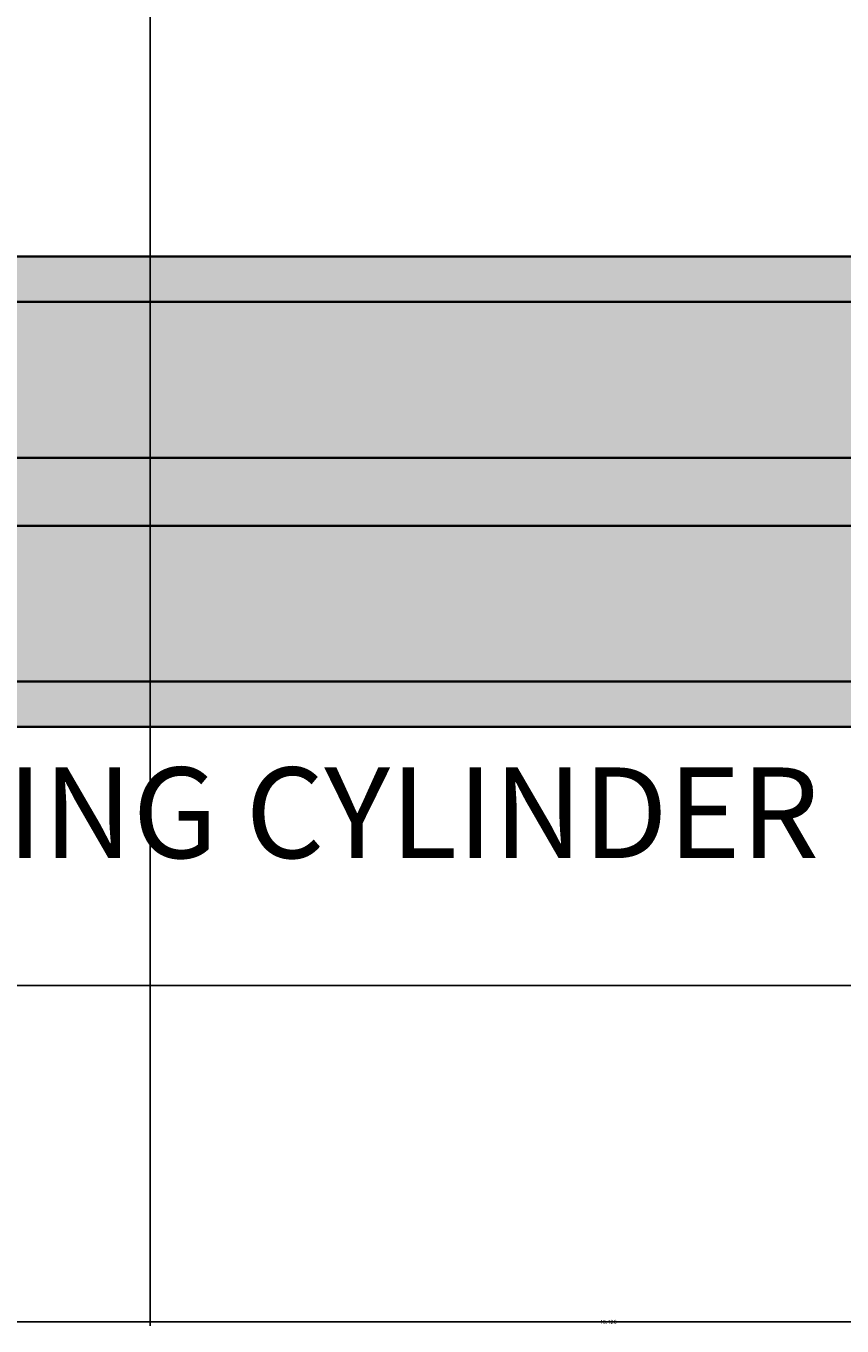
# Model space of a CAD drawing. Units: millimetres. Extents: x -11 to 280, y -4 to 208.
# Tile 28 of 55: x 186 to 222, y -4 to 54. Entities that reach past the tile are written whole.
import ezdxf

# ---------------------------------------------------------------- set-up
doc = ezdxf.new("R2010")
doc.units = ezdxf.units.MM
for name, color, linetype, lineweight in [('M-ANNO-TEXT', 7, 'Continuous', 18), ('M-DIMS', 2, 'Continuous', 18), ('M-HYDR-CYL', 7, 'Continuous', 35), ('M-HYDR-CYL-PATT', 252, 'Continuous', 13)]:
    doc.layers.add(name, color=color, linetype=linetype, lineweight=lineweight)
doc.styles.get("Standard").update_dxf_attribs({"font": 'arial.ttf'})
doc.dimstyles.get("Standard").update_dxf_attribs({"dimtxt": 0.18, "dimasz": 0.18, "dimexe": 0.18, "dimexo": 0.0625, "dimgap": 0.09, "dimtad": 0, "dimtih": 1, "dimtoh": 1, "dimdec": 4, "dimzin": 0, "dimdsep": 46, "dimtxsty": 'Standard', "dimcen": 0.09, "dimadec": 0, "dimazin": 0, "dimtfac": 1, "dimtdec": 4, "dimtofl": 0, "dimtmove": 0, "dimatfit": 3, "dimfxl": 1, "dimtolj": 1, "dimtzin": 0, "dimarcsym": 0})

# ---------------------------------------------------------------- blocks, each defined once
blk = doc.blocks.new('*D4')
at = {"layer": 'Defpoints', "color": 0, "transparency": 16777216}
for p in [(4.763, 84.426), (266.035, 51.733), (266.035, -3.415)]:
    blk.add_point(p, dxfattribs=at)
at = {"layer": 'M-DIMS', "color": 0, "lineweight": -2, "transparency": 16777216}
for p, q in [((4.763, 84.364), (4.763, -3.595)), ((266.035, 51.67), (266.035, -3.595)), ((4.943, -3.415), (134.934, -3.415)), ((265.855, -3.415), (135.864, -3.415))]:
    blk.add_line(p, q, dxfattribs=at)
at = {"layer": 'M-DIMS', "color": 0, "transparency": 16777216}
for points in [[(4.943, -3.385), (4.943, -3.445), (4.763, -3.415)], [(265.855, -3.385), (265.855, -3.445), (266.035, -3.415)]]:
    blk.add_solid(points, dxfattribs=at)
at = {"layer": 'M-DIMS', "color": 0, "transparency": 16777216, "insert": (135.399, -3.415), "char_height": 0.18, "attachment_point": 5}
blk.add_mtext('\\A1;261.27', dxfattribs=at)
blk = doc.blocks.new('*D5')
at = {"layer": 'Defpoints', "color": 0, "transparency": 16777216}
for p in [(24.759, 192.645), (-10.087, 11.435), (261.686, 11.435)]:
    blk.add_point(p, dxfattribs=at)
at = {"layer": 'M-DIMS', "color": 0, "lineweight": -2, "transparency": 16777216}
for p, q in [((24.696, 192.645), (-10.267, 192.645)), ((-10.087, 192.465), (-10.087, 102.222)), ((-10.087, 11.615), (-10.087, 101.858)), ((261.624, 11.435), (-10.267, 11.435))]:
    blk.add_line(p, q, dxfattribs=at)
at = {"layer": 'M-DIMS', "color": 0, "transparency": 16777216}
for points in [[(-10.117, 192.465), (-10.057, 192.465), (-10.087, 192.645)], [(-10.117, 11.615), (-10.057, 11.615), (-10.087, 11.435)]]:
    blk.add_solid(points, dxfattribs=at)
at = {"layer": 'M-DIMS', "color": 0, "transparency": 16777216, "insert": (-10.087, 102.04), "char_height": 0.18, "attachment_point": 5}
blk.add_mtext('\\A1;181.2', dxfattribs=at)
blk = doc.blocks.new('*D13')
at = {"layer": 'Defpoints', "color": 0, "transparency": 16777216}
for p in [(191.774, 105.314), (232.2, 105.314), (232.2, -3.415)]:
    blk.add_point(p, dxfattribs=at)
at = {"layer": 'M-DIMS', "color": 0, "lineweight": -2, "transparency": 16777216}
for p, q in [((191.774, 105.252), (191.774, -3.595)), ((232.2, 105.252), (232.2, -3.595)), ((191.954, -3.415), (211.52, -3.415)), ((232.02, -3.415), (212.454, -3.415))]:
    blk.add_line(p, q, dxfattribs=at)
at = {"layer": 'M-DIMS', "color": 0, "transparency": 16777216}
for points in [[(191.954, -3.385), (191.954, -3.445), (191.774, -3.415)], [(232.02, -3.385), (232.02, -3.445), (232.2, -3.415)]]:
    blk.add_solid(points, dxfattribs=at)
at = {"layer": 'M-DIMS', "color": 0, "transparency": 16777216, "insert": (211.987, -3.415), "char_height": 0.18, "attachment_point": 5}
blk.add_mtext('\\A1;40.426', dxfattribs=at)
blk = doc.blocks.new('*D20')
at = {"layer": 'Defpoints', "color": 0, "transparency": 16777216}
for p in [(231.68, 207.495), (151.022, 43.599), (231.68, 43.599)]:
    blk.add_point(p, dxfattribs=at)
at = {"layer": 'M-DIMS', "color": 0, "lineweight": -2, "transparency": 16777216}
for p, q in [((151.022, 43.662), (151.022, 207.675)), ((231.68, 43.662), (231.68, 207.675)), ((151.202, 207.495), (190.957, 207.495)), ((231.5, 207.495), (191.745, 207.495))]:
    blk.add_line(p, q, dxfattribs=at)
at = {"layer": 'M-DIMS', "color": 0, "transparency": 16777216}
for points in [[(151.202, 207.525), (151.202, 207.465), (151.022, 207.495)], [(231.5, 207.525), (231.5, 207.465), (231.68, 207.495)]]:
    blk.add_solid(points, dxfattribs=at)
at = {"layer": 'M-DIMS', "color": 0, "transparency": 16777216, "insert": (191.351, 207.495), "char_height": 0.18, "attachment_point": 5}
blk.add_mtext('\\A1;80.66', dxfattribs=at)

msp = doc.modelspace()

# ---------------------------------------------------------------- hatches: boundary and pattern name
at = {"layer": 'M-HYDR-CYL-PATT'}
h = msp.add_hatch(color=256, dxfattribs=at)
h.set_gradient(color1=(128, 128, 128), color2=(99, 100, 102), tint=1)
h.paths.add_polyline_path([(163.0955, 41.5991), (160.6935, 41.5991), (160.6935, 24.846), (163.0955, 24.846)])
h.paths.add_polyline_path([(259.871, 34.7226), (163.0955, 34.7226), (163.0955, 31.7226), (259.871, 31.7226, 1)])
h.paths.add_polyline_path([(257.0171, 42.0966), (265.5958, 50.6754, 1), (263.4745, 52.7967), (253.6316, 42.9537), (253.6316, 34.7226), (257.0171, 34.7226)])
h.paths.add_polyline_path([(257.0171, 25.6028), (257.0171, 31.7226), (253.6316, 31.7226), (253.6316, 26.785), (249.6456, 22.7991), (249.6456, 13.7204, 1), (252.6456, 13.7204), (252.6456, 21.2313)])
h.paths.add_polyline_path([(265.4334, 20.9382), (261.6863, 20.9382), (261.6863, 11.4346), (265.4334, 11.4346)])
h.paths.add_polyline_path([(261.6863, 17.1598), (252.6456, 17.1598), (252.6456, 15.9126), (261.6863, 15.9126)])
h = msp.add_hatch(color=256, dxfattribs=at)
h.set_gradient(color1=(102, 52, 60), color2=(102, 52, 60), tint=1)
h.paths.add_polyline_path([(153.0217, 24.846), (153.0217, 41.5991), (156.2446, 41.5991), (156.2446, 43.5991), (151.0217, 43.5991), (151.0217, 22.846), (231.6803, 22.846), (231.6803, 31.7226), (229.6803, 31.7226), (229.6803, 24.846)])
h.paths.add_polyline_path([(159.7446, 43.5991), (159.7446, 41.5991), (163.0955, 41.5991), (229.6803, 41.5991), (229.6803, 34.7226), (231.6803, 34.7226), (231.6803, 43.5991)], flags=17)
h = msp.add_hatch(color=256, dxfattribs=at)
h.set_gradient(color1=(76, 38, 47), color2=(34, 52, 110), tint=1, name='INVCYLINDER')
h.paths.add_polyline_path([(163.0955, 41.5991), (163.0955, 34.7226), (229.6803, 34.7226), (229.6803, 41.5991)])
h.paths.add_polyline_path([(229.6803, 24.846), (229.6803, 31.7226), (163.0955, 31.7226), (163.0955, 24.846)])

# ---------------------------------------------------------------- linework, layer by layer
at = {"layer": 'M-HYDR-CYL'}
for p, q in [((259.871, 34.7226), (163.0955, 34.7226)), ((259.871, 31.7226), (163.0955, 31.7226))]:
    msp.add_line(p, q, dxfattribs=at)
for points in [[(231.6803, 31.7226), (231.6803, 22.846), (151.0217, 22.846), (151.0217, 43.5991), (156.2446, 43.5991)], [(159.7446, 43.5991), (231.6803, 43.5991), (231.6803, 34.7226)], [(229.6803, 31.7226), (229.6803, 24.846), (153.0217, 24.846), (153.0217, 41.5991), (156.2446, 41.5991)], [(159.7446, 41.5991), (229.6803, 41.5991), (229.6803, 34.7226)]]:
    msp.add_lwpolyline(points, dxfattribs=at)

# ---------------------------------------------------------------- texts
at = {"layer": 'M-ANNO-TEXT', "insert": (164.865, 21.0543), "char_height": 4, "attachment_point": 1}
msp.add_mtext_dynamic_manual_height_columns('ACTUATING CYLINDER', width=63.617875, gutter_width=12.5, heights=[0], dxfattribs=at)

# ---------------------------------------------------------------- dimensions: what is measured, and where the dimension line sits
at = {"layer": 'M-DIMS'}
for base, p1, p2, override, picture, middle in [((231.6803, 207.495), (151.0217, 43.5991), (231.6803, 43.5991), {"dimdec": 2, "dimlfac": 1, "dimrnd": 0, "dimzin": 0, "dimdsep": 46, "dimlunit": 2}, '*D20', (191.351, 207.495)), ((232.20002, -3.41542), (191.77448, 105.31407), (232.20002, 105.31407), {"dimdec": 3, "dimlfac": 1, "dimrnd": 0, "dimzin": 0, "dimdsep": 46, "dimlunit": 2}, '*D13', (211.98725, -3.41542)), ((266.0352, -3.4154), (4.7635, 84.4261), (266.0352, 51.7328), {"dimdec": 2, "dimlfac": 1, "dimrnd": 0, "dimzin": 0, "dimdsep": 46, "dimlunit": 2}, '*D4', (135.3993, -3.4154))]:
    dim = msp.add_linear_dim(base=base, p1=p1, p2=p2, dimstyle='Standard', override=override, dxfattribs=at)
    dim.commit()
    dim.dimension.update_dxf_attribs({"geometry": picture, "text_midpoint": middle})
dim = msp.add_linear_dim(base=(-10.0865, 11.4346), p1=(24.7588, 192.645), p2=(261.6863, 11.4346), angle=90, dimstyle='Standard', override={"dimdec": 1, "dimlfac": 1, "dimrnd": 0, "dimzin": 0, "dimdsep": 46, "dimlunit": 2}, dxfattribs=at)
dim.commit()
dim.dimension.update_dxf_attribs({"geometry": '*D5', "text_midpoint": (-10.0865, 102.0398)})

doc.saveas('drawing.dxf')
